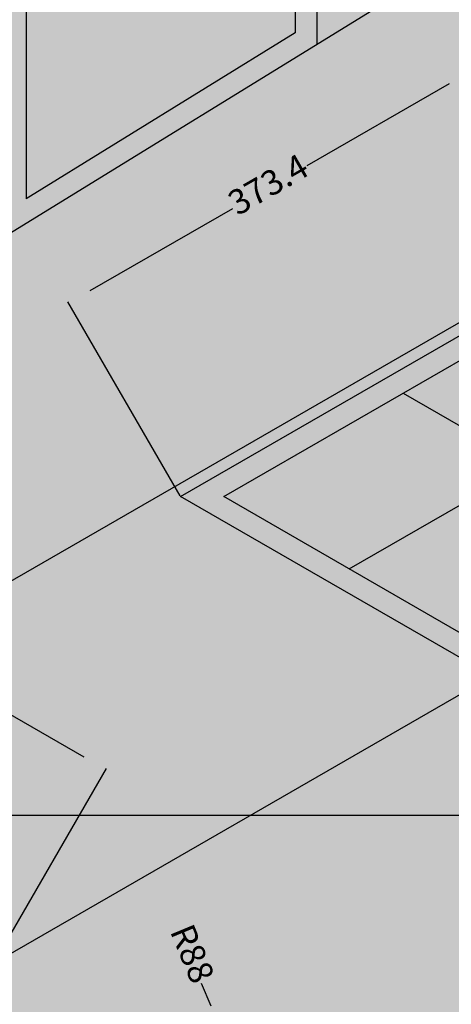
# Model space of a CAD drawing. Units: millimetres. Extents: x 78378 to 86415, y 148682 to 152721.
# Tile 3 of 18: x 78851 to 79199, y 149702 to 150495. Entities that reach past the tile are written whole.
import ezdxf

# ---------------------------------------------------------------- set-up
doc = ezdxf.new("R2010")
doc.units = ezdxf.units.MM
for name, color, linetype, lineweight in [('A-ANNO-DIMS', 2, 'Continuous', 18), ('A-FURN', 4, 'Continuous', 25), ('A-FURN-PATT', 32, 'Continuous', 13)]:
    doc.layers.add(name, color=color, linetype=linetype, lineweight=lineweight)
doc.styles.get("Standard").update_dxf_attribs({"font": 'arial.ttf'})
doc.dimstyles.new('ISO-25', dxfattribs={"dimtxt": 20, "dimasz": 20, "dimexe": 1.25, "dimexo": 0.625, "dimtad": 0, "dimdec": 1, "dimtxsty": 'Standard', "dimcen": 2.5, "dimadec": 0, "dimazin": 0, "dimtfac": 1, "dimtdec": 1, "dimtmove": 0, "dimatfit": 3, "dimfxl": 1, "dimarcsym": 0})

# ---------------------------------------------------------------- blocks, each defined once
blk = doc.blocks.new('*D19')
at = {"layer": 'A-ANNO-DIMS', "color": 0, "lineweight": -2, "transparency": 16777216}
for p, q in [((78571.17, 149885.55), (78661.48, 150041.97)), ((78678.18, 150030.89), (78771.12, 149977.23)), ((78903.35, 149900.89), (78810.4, 149954.55)), ((78830.98, 149735.55), (78921.29, 149891.97))]:
    blk.add_line(p, q, dxfattribs=at)
at = {"layer": 'A-ANNO-DIMS', "color": 0, "transparency": 16777216}
for points in [[(78679.85, 150033.78), (78676.51, 150028.01), (78660.86, 150040.89)], [(78905.01, 149903.78), (78901.68, 149898.01), (78920.67, 149890.89)]]:
    blk.add_solid(points, dxfattribs=at)
at = {"layer": 'Defpoints', "color": 0, "transparency": 16777216}
for p in [(78920.67, 149890.89), (78570.86, 149885.01), (78830.67, 149735.01)]:
    blk.add_point(p, dxfattribs=at)
at = {"layer": 'A-ANNO-DIMS', "color": 0, "transparency": 16777216, "insert": (78790.76, 149965.89), "char_height": 20, "attachment_point": 5, "rotation": 330}
blk.add_mtext('300', dxfattribs=at)
blk = doc.blocks.new('*D23')
at = {"layer": 'A-ANNO-DIMS', "color": 0, "lineweight": -2, "transparency": 16777216}
for p, q in [((79304.01, 150298.13), (79213.69, 150454.55)), ((79197, 150443.47), (79082.34, 150377.27)), ((78908.24, 150276.76), (79022.89, 150342.95)), ((78980.6, 150111.41), (78890.29, 150267.84))]:
    blk.add_line(p, q, dxfattribs=at)
at = {"layer": 'A-ANNO-DIMS', "color": 0, "transparency": 16777216}
for points in [[(79195.33, 150446.36), (79198.67, 150440.59), (79214.32, 150453.47)], [(78906.57, 150279.64), (78909.9, 150273.87), (78890.92, 150266.76)]]:
    blk.add_solid(points, dxfattribs=at)
at = {"layer": 'Defpoints', "color": 0, "transparency": 16777216}
for p in [(79214.32, 150453.47), (79304.32, 150297.59), (78980.92, 150110.87)]:
    blk.add_point(p, dxfattribs=at)
at = {"layer": 'A-ANNO-DIMS', "color": 0, "transparency": 16777216, "insert": (79052.62, 150360.11), "char_height": 20, "attachment_point": 5, "rotation": 30}
blk.add_mtext('373.4', dxfattribs=at)
blk = doc.blocks.new('*D25')
at = {"layer": 'A-ANNO-DIMS', "color": 0, "lineweight": -2, "transparency": 16777216}
for p, q in [((79360.48, 149854.03), (78389.61, 149854.03)), ((78390.86, 149834.03), (78390.86, 149656.62)), ((78390.86, 149409.86), (78390.86, 149587.28)), ((79360.48, 149389.86), (78389.61, 149389.86))]:
    blk.add_line(p, q, dxfattribs=at)
at = {"layer": 'A-ANNO-DIMS', "color": 0, "transparency": 16777216}
for points in [[(78387.53, 149834.03), (78394.19, 149834.03), (78390.86, 149854.03)], [(78387.53, 149409.86), (78394.19, 149409.86), (78390.86, 149389.86)]]:
    blk.add_solid(points, dxfattribs=at)
at = {"layer": 'Defpoints', "color": 0, "transparency": 16777216}
for p in [(78390.86, 149854.03), (79361.1, 149854.03), (79361.1, 149389.86)]:
    blk.add_point(p, dxfattribs=at)
at = {"layer": 'A-ANNO-DIMS', "color": 0, "transparency": 16777216, "insert": (78390.86, 149621.95), "char_height": 20, "attachment_point": 5, "rotation": 90}
blk.add_mtext('464.2', dxfattribs=at)
blk = doc.blocks.new('*D61')
at = {"layer": 'A-ANNO-DIMS', "color": 0, "lineweight": -2, "transparency": 16777216}
for p, q in [((79224.25, 149639.59), (79209.69, 149625.87)), ((79095.12, 149517.87), (79195.14, 149612.15))]:
    blk.add_line(p, q, dxfattribs=at)
at = {"layer": 'A-ANNO-DIMS', "color": 0, "transparency": 16777216}
blk.add_solid([(79207.41, 149628.29), (79211.98, 149623.44), (79195.14, 149612.15)], dxfattribs=at)
at = {"layer": 'Defpoints', "color": 0, "transparency": 16777216}
for p in [(79195.14, 149612.15), (79095.12, 149517.87)]:
    blk.add_point(p, dxfattribs=at)
at = {"layer": 'A-ANNO-DIMS', "color": 0, "transparency": 16777216, "insert": (79261.93, 149675.1), "char_height": 20, "attachment_point": 5, "rotation": 43.30618}
blk.add_mtext('R137.45', dxfattribs=at)
blk = doc.blocks.new('*D62')
at = {"layer": 'A-ANNO-DIMS', "color": 0, "lineweight": -2, "transparency": 16777216}
for p, q in [((78997.43, 149719.03), (79005.1, 149700.56)), ((79046.52, 149600.81), (79012.77, 149682.09))]:
    blk.add_line(p, q, dxfattribs=at)
at = {"layer": 'A-ANNO-DIMS', "color": 0, "transparency": 16777216}
blk.add_solid([(79008.18, 149701.84), (79002.02, 149699.28), (79012.77, 149682.09)], dxfattribs=at)
at = {"layer": 'Defpoints', "color": 0, "transparency": 16777216}
for p in [(79012.77, 149682.09), (79046.52, 149600.81)]:
    blk.add_point(p, dxfattribs=at)
at = {"layer": 'A-ANNO-DIMS', "color": 0, "transparency": 16777216, "insert": (78988.02, 149741.69), "char_height": 20, "attachment_point": 5, "rotation": 292.54744}
blk.add_mtext('R88', dxfattribs=at)

msp = doc.modelspace()

# ---------------------------------------------------------------- hatches: boundary and pattern name
at = {"layer": 'A-FURN-PATT'}
h = msp.add_hatch(color=256, dxfattribs=at)
h.dxf.hatch_style = 1
h.paths.add_polyline_path([(78839.3276, 151040.0076), (78579.52, 151190.0076), (78579.52, 150470.0076), (78839.3276, 150320.0076)])
h.paths.add_polyline_path([(79073.1545, 150899.6469, 0.27777969), (79002.2645, 150996.3205, 0.79108393), (78917.9567, 150978.8719, 0.18044832), (78856.6481, 150853.0138), (78856.6481, 150350.6973), (79073.1545, 150484.318)])
h.paths.add_polyline_path([(79073.1545, 151175.0076), (78856.6481, 151050.0076), (78856.6481, 150853.0138, -0.18044832), (78917.9567, 150978.8719, -0.79108393), (79002.2645, 150996.3205, -0.27777969), (79073.1545, 150899.6469)])
h.paths.add_polyline_path([(79341.6224, 151350.0076), (79099.1352, 151490.0076), (78596.8405, 151200.0076), (78839.3276, 151060.0076)])
h.paths.add_polyline_path([(79904.5389, 151675.0076), (79662.0518, 151815.0076), (79099.1352, 151490.0076), (79341.6224, 151350.0076)])
h.paths.add_polyline_path([(80389.5131, 151955.0076), (80389.5131, 152235.0076), (79662.0518, 151815.0076), (79904.5389, 151675.0076)])
h.paths.add_polyline_path([(80389.5131, 151955.0076), (80164.3465, 151825.0076), (80164.3465, 151105.0076), (80614.6797, 151105.0076), (80614.6797, 151825.0076)])
edge = h.paths.add_edge_path(flags=16)
edge.add_spline(control_points=[(80216.308, 151728.251), (80227.1854, 151732.981), (80256.3301, 151745.6544), (80298.41, 151761.9595), (80340.2597, 151805.855), (80391.0771, 151782.0404), (80454.0396, 151805.7581), (80496.5007, 151742.4095), (80543.8218, 151733.4043), (80562.7182, 151729.8083)], knot_values=[0, 0, 0, 0, 35.54374676, 95.23575347, 136.36767513, 200.93298197, 236.72641081, 322.88993498, 380.17027367, 380.17027367, 380.17027367, 380.17027367], degree=3, periodic=0)
edge.add_line((80562.7182, 151729.8083), (80562.7182, 151165.0076))
edge.add_line((80562.7182, 151165.0076), (80216.308, 151165.0076))
edge.add_line((80216.308, 151165.0076), (80216.308, 151728.251))
h.paths.add_polyline_path([(80632.0002, 152095.0076), (80389.5131, 152235.0076), (80389.5131, 151955.0076), (80614.6797, 151825.0076), (80632.0002, 151815.0076)])
h.paths.add_polyline_path([(80867.7794, 151958.8805), (80632.0002, 152095.0076), (80632.0002, 151815.0076), (80632.0002, 151510.0076), (80867.7794, 151373.8805)])
h.paths.add_polyline_path([(80147.026, 151495.8203, 0.18918979), (80063.5671, 151597.7244, 0.78826136), (79979.2691, 151580.5832, 0.16072613), (79904.5389, 151413.5769), (79904.5389, 150955.0076), (80147.026, 151095.0076)])
h.paths.add_polyline_path([(80147.026, 151815.0076), (79904.5389, 151675.0076), (79904.5389, 151413.5769, -0.16072613), (79979.2691, 151580.5832, -0.78826136), (80063.5671, 151597.7244, -0.18918979), (80147.026, 151495.8203)])
h.paths.add_polyline_path([(79887.2184, 151645.0076), (79640.4011, 151502.5076), (79640.4011, 151262.3325, -0.16072613), (79715.1313, 151429.3387, -0.78826136), (79799.4294, 151446.48, -0.21290578), (79887.2184, 151328.7247)])
h.paths.add_polyline_path([(79799.4294, 151446.48, 0.78826136), (79715.1313, 151429.3387, 0.16072613), (79640.4011, 151262.3325), (79640.4011, 150822.5076), (79887.2184, 150965.0076), (79887.2184, 151328.7247, 0.21290578)])
h.paths.add_polyline_path([(79605.7601, 151482.5076), (79358.9429, 151340.0076), (79358.9429, 151100.0701, -0.16072613), (79433.6731, 151267.0764, -0.78826136), (79517.9711, 151284.2176, -0.21290578), (79605.7601, 151166.4623)])
h.paths.add_polyline_path([(79605.7601, 151166.4623, 0.21290578), (79517.9711, 151284.2176, 0.78826136), (79433.6731, 151267.0764, 0.16072613), (79358.9429, 151100.0701), (79358.9429, 150742.9831), (79419.0877, 150694.7323), (79605.7601, 150802.5076)])
edge = h.paths.add_edge_path(flags=0)
edge.add_spline(control_points=[(81152.4356, 151098.7676), (81105.7208, 151145.9466), (81038.6136, 151213.7208), (80882.3866, 151214.1938), (80797.4434, 151311.2997), (80711.8686, 151340.3754), (80681.7691, 151350.6023)], knot_values=[0, 0, 0, 0, 188.233441, 270.4032752, 445.45179201, 540.42858829, 540.42858829, 540.42858829, 540.42858829], degree=3, periodic=0)
edge.add_line((80683.4538, 151350.0269), (80683.4538, 151104.8792))
edge.add_line((80683.4538, 151104.8792), (81152.4356, 150851.399))
edge.add_line((81152.4356, 150851.399), (81152.4356, 151098.7676))
edge = h.paths.add_edge_path(flags=0)
edge.add_spline(control_points=[(80912.9018, 151027.1103), (80892.3742, 151034.1027), (80860.1663, 151045.0739), (80835.5097, 151068.1214), (80826.5679, 151076.4797)], knot_values=[0, 0, 0, 0, 63.98405104, 100.39142428, 100.39142428, 100.39142428, 100.39142428], degree=3, periodic=0)
edge.add_arc((80830.0414, 151081.2992), 5.9407, 100.9277276, 234.2187381, ccw=False)
edge.add_spline(control_points=[(80828.9152, 151087.1322), (80837.857, 151078.7739), (80862.5136, 151055.7263), (80894.7215, 151044.7552), (80915.2491, 151037.7628)], knot_values=[0, 0, 0, 0, 36.40737324, 100.39142428, 100.39142428, 100.39142428, 100.39142428], degree=3, periodic=0)
edge.add_arc((80914.7882, 151032.2795), 5.5026, -107.9540399, 85.195579, ccw=False)
h.paths.add_polyline_path([(81238.218, 151110.0076), (80632.0002, 151460.0076), (80632.0002, 151105.0076), (81238.218, 150755.0076)])
edge = h.paths.add_edge_path(flags=16)
edge.add_line((81152.4356, 150851.399), (80683.4538, 151104.8792))
edge.add_line((80683.4538, 151104.8792), (80683.4538, 151350.0279))
edge.add_spline(control_points=[(80681.7691, 151350.6023), (80711.8686, 151340.3754), (80797.4434, 151311.2997), (80882.3866, 151214.1938), (81038.6136, 151213.7208), (81105.7208, 151145.9466), (81152.4356, 151098.7676)], knot_values=[0, 0, 0, 0, 94.97679628, 270.02531309, 352.19514729, 540.42858829, 540.42858829, 540.42858829, 540.42858829], degree=3, periodic=0)
edge.add_line((81152.4356, 151098.7676), (81152.4356, 150851.399))
edge = h.paths.add_edge_path(flags=0)
edge.add_spline(control_points=[(80912.9018, 151027.1103), (80892.3742, 151034.1027), (80860.1663, 151045.0739), (80835.5097, 151068.1214), (80826.5679, 151076.4797)], knot_values=[0, 0, 0, 0, 63.98405104, 100.39142428, 100.39142428, 100.39142428, 100.39142428], degree=3, periodic=0)
edge.add_arc((80830.0414, 151081.2992), 5.9407, 100.9277276, 234.2187381, ccw=False)
edge.add_spline(control_points=[(80828.9152, 151087.1322), (80837.857, 151078.7739), (80862.5136, 151055.7263), (80894.7215, 151044.7552), (80915.2491, 151037.7628)], knot_values=[0, 0, 0, 0, 36.40737324, 100.39142428, 100.39142428, 100.39142428, 100.39142428], degree=3, periodic=0)
edge.add_arc((80914.7882, 151032.2795), 5.5026, -107.7417882, 85.195579, ccw=False)
h.paths.add_polyline_path([(81498.0256, 151255.0076), (81238.218, 151110.0076), (81238.218, 150755.0076), (81498.0256, 150905.0076)])
edge = h.paths.add_edge_path(flags=16)
edge.add_spline(control_points=[(81152.4356, 151098.7676), (81105.7208, 151145.9466), (81038.6136, 151213.7208), (80882.3866, 151214.1938), (80797.4434, 151311.2997), (80711.8686, 151340.3754), (80681.7691, 151350.6023)], knot_values=[0, 0, 0, 0, 188.233441, 270.4032752, 445.45179201, 540.42858829, 540.42858829, 540.42858829, 540.42858829], degree=3, periodic=0)
edge.add_line((80683.4538, 151350.0279), (80683.4538, 151104.8792))
edge.add_line((80683.4538, 151104.8792), (81152.4356, 150851.399))
edge.add_line((81152.4356, 150851.399), (81152.4356, 151098.7676))
h.paths.add_polyline_path([(81453.9904, 151280.4314), (80867.7794, 151618.8805), (80867.7794, 151373.8805), (81238.218, 151160.0076)])
edge = h.paths.add_edge_path(flags=16)
edge.add_line((81189.2304, 151297.6373), (81114.4166, 151300.2154))
edge.add_arc((81412.0967, 151394.0167), 312.1092, 179.7569303, 197.4900342, ccw=False)
edge.add_ellipse((81154.0183, 151392.0436), major_axis=(-54.0264, 3.6301), ratio=0.22179693, start_angle=0, end_angle=0.3517985, ccw=False)
edge.add_ellipse((81154.0183, 151392.0436), major_axis=(-54.0264, 3.6301), ratio=0.22179693, start_angle=180, end_angle=360, ccw=False)
edge.add_spline(control_points=[(81196.1844, 151321.9476), (81224.9802, 151347.1455), (81266.8846, 151383.8144), (81222.0354, 151387.0304), (81208.0056, 151388.0364)], knot_values=[0, 0, 0, 0, 75.09175173, 109.27580439, 109.27580439, 109.27580439, 109.27580439], degree=3, periodic=0)
edge.add_arc((80751.9112, 151435.6145), 458.5693, 342.4891602, 345.646172, ccw=False)
edge = h.paths.add_edge_path(flags=0)
edge.add_spline(control_points=[(81196.6193, 151323.657), (81197.893, 151324.7717), (81199.1654, 151325.8858), (81209.0233, 151334.5343), (81217.3959, 151341.9835), (81228.0928, 151352.5012), (81231.3883, 151355.9524), (81236.9493, 151362.4395), (81239.214, 151365.4773), (81241.4987, 151369.416), (81242.064, 151370.5542), (81242.9187, 151372.6971), (81243.2076, 151373.7015), (81243.5012, 151375.5539), (81243.5065, 151376.4), (81243.2432, 151377.9407), (81242.9775, 151378.6373), (81242.1402, 151379.937), (81241.5659, 151380.5416), (81240.2039, 151381.533), (81239.4963, 151381.9384), (81237.0619, 151383.0663), (81235.0242, 151383.6999), (81230.352, 151384.7569), (81227.7173, 151385.1826), (81221.9118, 151385.9145), (81218.7193, 151386.2133), (81213.7912, 151386.6115), (81212.1252, 151386.7359), (81209.6196, 151386.9181), (81208.7865, 151386.9779), (81207.9009, 151387.0432)], knot_values=[0.01548744, 0.01548744, 0.01548744, 0.01548744, 3.33787957, 3.33787957, 25.85130624, 25.85130624, 37.52811308, 37.52811308, 49.20491992, 49.20491992, 54.2850938, 54.2850938, 59.36526768, 59.36526768, 64.44544157, 64.44544157, 69.52561545, 69.52561545, 74.60578933, 74.60578933, 78.49366785, 78.49366785, 86.25567095, 86.25567095, 94.01767406, 94.01767406, 102.20226556, 102.20226556, 106.29456131, 106.29456131, 108.32522175, 108.32522175, 108.32522175, 108.32522175], degree=3, periodic=0)
edge = h.paths.add_edge_path(flags=16)
edge.add_arc((81034.1732, 151350.4693), 42.5822, 231.2679035, 306.151846, ccw=False)
edge.add_line((81007.5303, 151317.2517), (81007.5303, 151395.181))
edge.add_ellipse((81033.412, 151394.7791), major_axis=(-25.8816, 0.4538), ratio=0.23894509, start_angle=0, end_angle=0.1147075, ccw=False)
edge.add_ellipse((81033.412, 151394.7791), major_axis=(-25.8816, 0.4538), ratio=0.23894509, start_angle=181.1677709, end_angle=358.9476457, ccw=False)
edge.add_ellipse((81033.412, 151395.7791), major_axis=(-25.8816, 0.4538), ratio=0.23894509, start_angle=180, end_angle=360.1147075, ccw=False)
edge.add_ellipse((81033.412, 151395.7791), major_axis=(-25.8816, 0.4538), ratio=0.23894509, start_angle=178.9476457, end_angle=180, ccw=False)
edge.add_line((81059.2936, 151395.1778), (81059.2936, 151394.3772))
edge.add_ellipse((81033.412, 151394.7791), major_axis=(-25.8816, 0.4538), ratio=0.23894509, start_angle=180, end_angle=180.1147075, ccw=False)
edge.add_ellipse((81033.412, 151394.7791), major_axis=(-25.8816, 0.4538), ratio=0.23894509, start_angle=3.6903098, end_angle=176.4406503, ccw=False)
edge.add_line((81059.2936, 151393.3388), (81059.2936, 151316.086))
h.paths.add_polyline_path([(80951.9355, 151343.9568), (80909.6838, 151362.4635), (80904.0219, 151443.9615, -0.38133308), (80987.2169, 151411.3717)], flags=16)
h = msp.add_hatch(color=256, dxfattribs=at)
h.dxf.hatch_style = 1
h.paths.add_polyline_path([(80389.8136, 150935.1811), (80389.5131, 151105.0076), (80164.3465, 151105.0076), (79904.5389, 150955.0076), (79433.5848, 150683.1022), (79459.4128, 150662.3818), (79243.9048, 150537.9582), (79160.4069, 150518.1674), (78839.3276, 150320.0076), (78579.52, 150470.0076), (78570.8597, 150475.0076), (78570.8597, 150465.0076), (78570.8597, 149885.0076)])
h.paths.add_polyline_path([(80086.4042, 150460.0076), (79826.5966, 150610.0076), (78570.8597, 149885.0076), (78830.6674, 149735.0076)])
h.paths.add_polyline_path([(79540.8001, 150161.0557), (79217.3967, 149974.3386), (78980.9166, 150110.8705), (79304.32, 150297.5875)], flags=16)
h.paths.add_polyline_path([(79506.159, 150161.0557), (79217.3967, 149994.3386), (79015.5576, 150110.8705), (79304.32, 150277.5875)], flags=0)
edge = h.paths.add_edge_path(flags=0)
edge.add_arc((79247.8636, 150177.1541), 137.9799, 256.0025928, 293.5594109)
edge.add_arc((79240.7671, 150078.2605), 68.0855, 336.099104, 387.3696877)
edge.add_ellipse((79258.3074, 150109.4852), major_axis=(-42.6234, -1.6591), ratio=0.16042843, start_angle=0, end_angle=179.0977279, ccw=False)
edge.add_arc((79285.2112, 150074.2509), 77.2096, 155.1233104, 203.6557939)
edge = h.paths.add_edge_path(flags=0)
edge.add_ellipse((79258.6958, 150110.8297), major_axis=(-42.6234, -1.6591), ratio=0.16042843, start_angle=350.6039412, end_angle=356.2289762)
edge.add_line((79219.169, 150111.8937), (79218.3268, 150109.4141))
edge.add_arc((79262.4675, 150032.9602), 88.2813, 112.3931229, 120, ccw=False)
h.paths.add_polyline_path([(79287.0625, 150086.9703, -0.24770206), (79288.1967, 150077.2955, -0.39047651), (79265.4731, 150072.5438, -0.48726153), (79264.079, 150082.3769, 0.39560433)], flags=0)
h.paths.add_polyline_path([(80389.5131, 150935.0076), (79826.5966, 150610.0076), (80086.4042, 150460.0076), (80692.622, 150460.0076), (80952.4296, 150610.0076)])
edge = h.paths.add_edge_path(flags=16)
edge.add_ellipse((80392.4466, 150825.601), major_axis=(-133.0757, 7.722), ratio=0.42449957, start_angle=0, end_angle=360)
edge = h.paths.add_edge_path(flags=0)
edge.add_spline(control_points=[(80269.3541, 150832.7436), (80269.2919, 150831.672), (80269.3503, 150830.5922), (80269.7341, 150828.3361), (80270.0612, 150827.1587), (80271.0461, 150824.6748), (80271.7052, 150823.3692), (80273.4061, 150820.6503), (80274.4481, 150819.2381), (80276.9366, 150816.3509), (80278.3828, 150814.8762), (80282.5858, 150811.0913), (80285.6261, 150808.7701), (80292.6031, 150804.2267), (80296.5388, 150802.0041), (80305.195, 150797.7581), (80309.9151, 150795.7344), (80320.0112, 150791.96), (80325.387, 150790.2092), (80339.2162, 150786.315), (80347.9578, 150784.3563), (80366.0679, 150781.2568), (80375.4359, 150780.1158), (80394.3093, 150778.7158), (80403.8142, 150778.4568), (80422.4656, 150778.8319), (80431.6115, 150779.4662), (80449.0608, 150781.5838), (80457.3636, 150783.0675), (80472.6699, 150786.7766), (80479.6726, 150789.0033), (80490.1894, 150793.2813), (80494.1268, 150795.1967), (80501.0146, 150799.1885), (80503.9632, 150801.2651), (80508.2066, 150804.9015), (80509.73, 150806.4609), (80512.1996, 150809.4942), (80513.1456, 150810.9657), (80514.4291, 150813.5431), (80514.8436, 150814.6688), (80515.3984, 150816.8625), (80515.5405, 150817.9315), (80515.5801, 150820.098), (80515.4773, 150821.1978), (80514.9905, 150823.5062), (80514.6047, 150824.7154), (80513.4854, 150827.2641), (80512.7511, 150828.6027), (80510.8872, 150831.3809), (80509.7578, 150832.8196), (80507.0873, 150835.7513), (80505.5466, 150837.2439), (80501.0624, 150841.0944), (80497.8199, 150843.4576), (80490.4174, 150848.062), (80486.2582, 150850.3037), (80477.1448, 150854.5643), (80472.1909, 150856.5835), (80461.6275, 150860.3245), (80456.0182, 150862.0465), (80441.7332, 150865.8127), (80432.7885, 150867.6675), (80414.3391, 150870.5317), (80404.8349, 150871.5411), (80385.7707, 150872.6572), (80376.2113, 150872.764), (80357.5444, 150872.0728), (80348.4375, 150871.2748), (80331.1682, 150868.83), (80323.0064, 150867.1827), (80309.472, 150863.5363), (80303.8628, 150861.6593), (80293.8018, 150857.5401), (80289.3512, 150855.2969), (80282.7757, 150851.2345), (80280.3473, 150849.4579), (80276.2606, 150845.9127), (80274.604, 150844.1458), (80272.3157, 150841.1243), (80271.5358, 150839.8454), (80270.3496, 150837.3879), (80269.9417, 150836.2101), (80269.5065, 150834.2815), (80269.3988, 150833.5143), (80269.3541, 150832.7436)], knot_values=[0, 0, 0, 0, 0.09750046, 0.09750046, 0.19500092, 0.19500092, 0.29250138, 0.29250138, 0.39000184, 0.39000184, 0.4875023, 0.4875023, 0.63880322, 0.63880322, 0.79010415, 0.79010415, 0.94140507, 0.94140507, 1.092706, 1.092706, 1.3128171, 1.3128171, 1.5329282, 1.5329282, 1.7530393, 1.7530393, 1.97315041, 1.97315041, 2.19326151, 2.19326151, 2.41337261, 2.41337261, 2.56986063, 2.56986063, 2.72634866, 2.72634866, 2.84418658, 2.84418658, 2.96202451, 2.96202451, 3.06023388, 3.06023388, 3.15844325, 3.15844325, 3.25665261, 3.25665261, 3.35486198, 3.35486198, 3.45307135, 3.45307135, 3.55128072, 3.55128072, 3.64949009, 3.64949009, 3.80392773, 3.80392773, 3.95836537, 3.95836537, 4.11280301, 4.11280301, 4.26724064, 4.26724064, 4.48920349, 4.48920349, 4.71116635, 4.71116635, 4.9331292, 4.9331292, 5.15509205, 5.15509205, 5.3770549, 5.3770549, 5.55785361, 5.55785361, 5.73865232, 5.73865232, 5.87239556, 5.87239556, 6.00613879, 6.00613879, 6.109605, 6.109605, 6.2130712, 6.2130712, 6.28318531, 6.28318531, 6.28318531, 6.28318531], degree=3, periodic=0)
edge = h.paths.add_edge_path(flags=0)
edge.add_ellipse((80392.4466, 150825.601), major_axis=(-101.8398, 3.3923), ratio=0.40349248, start_angle=0, end_angle=360)
edge = h.paths.add_edge_path(flags=0)
edge.add_ellipse((80391.1657, 150858.3746), major_axis=(9.0882, -0.6733), ratio=0.35135413, start_angle=0, end_angle=360)
h.paths.add_polyline_path([(80952.4296, 150610.0076), (80692.622, 150460.0076), (81361.2342, 150073.9842), (81649.9628, 150052.7286), (81766.4935, 150120.0076), (81766.4935, 150140.0076), (81564.9025, 150256.3963), (81564.8884, 150096.1963), (81538.9076, 150111.1963), (81538.9217, 150271.3963)])
h.paths.add_polyline_path([(81539.0357, 151571.3305), (80867.7794, 151958.8805), (80867.7794, 151618.8805), (81498.0256, 151255.0076), (81498.0256, 150905.0076), (81238.218, 150755.0076), (81538.9488, 150581.3806)])
h.paths.add_polyline_path([(81766.4935, 151440.0076), (81565.0164, 151556.3305), (81564.9296, 150566.3806), (81766.4935, 150450.0076)])
edge = h.paths.add_edge_path()
edge.add_line((81564.9296, 150566.3806), (81564.9137, 150384.6289))
edge.add_ellipse((81552.1304, 150358.5718), major_axis=(52.6272, 3.506), ratio=0.49589905, start_angle=367.5169757, end_angle=420.0564686, ccw=False)
edge.add_ellipse((81552.1304, 150358.5718), major_axis=(52.6272, 3.506), ratio=0.49589905, start_angle=351.729742, end_angle=367.5169757, ccw=False)
edge.add_ellipse((81552.1304, 150345.5016), major_axis=(52.6272, 3.506), ratio=0.49589905, start_angle=352.5116949, end_angle=366.3006092, ccw=False)
edge.add_line((81603.4463, 150342.2039), (81603.5064, 150340.4475))
edge.add_ellipse((81552.1304, 150332.128), major_axis=(52.6272, 3.506), ratio=0.49589905, start_angle=353.6729654, end_angle=365.3867997, ccw=False)
edge.add_ellipse((81552.1304, 150332.128), major_axis=(52.6272, 3.506), ratio=0.49589905, start_angle=350.9388331, end_angle=353.6729654)
edge.add_line((81603.8688, 150329.855), (81604.0442, 150324.7302))
edge.add_ellipse((81552.1304, 150317.7418), major_axis=(52.6272, 3.506), ratio=0.49589905, start_angle=355.2176746, end_angle=363.8553364, ccw=False)
edge.add_ellipse((81552.1304, 150317.7418), major_axis=(52.6272, 3.506), ratio=0.49589905, start_angle=341.3250873, end_angle=355.2176746, ccw=False)
edge.add_ellipse((81552.1304, 150317.7418), major_axis=(52.6272, 3.506), ratio=0.49589905, start_angle=293.4661701, end_angle=341.3250873, ccw=False)
edge.add_line((81564.9057, 150292.9664), (81564.9025, 150256.3963))
edge.add_line((81564.9025, 150256.3963), (81766.4935, 150140.0076))
edge.add_line((81766.4935, 150140.0076), (81766.4935, 150450.0076))
edge.add_line((81766.4935, 150450.0076), (81564.9296, 150566.3806))
h.paths.add_polyline_path([(81525.5713, 150321.598), (81526.5985, 150321.3069), (81528.6771, 150320.947)])
h.paths.add_polyline_path([(81512.7903, 150326.1129), (81514.5058, 150325.3887), (81512.538, 150326.2678)])
h.paths.add_polyline_path([(81533.2148, 150320.1615), (81534.6952, 150319.9052), (81536.5995, 150319.7557)])
h.paths.add_polyline_path([(81518.622, 150323.6513), (81519.227, 150323.3959), (81521.289, 150322.8116)])
h.paths.add_polyline_path([(81501.2183, 150336.2599), (81500.3543, 150338.1339), (81499.7815, 150340.0494), (81499.5032, 150341.9955), (81499.5032, 150343.7257), (81499.7584, 150345.5905), (81500.2766, 150347.4549), (81501.0551, 150349.3095), (81501.0967, 150349.3937), (81501.1389, 150349.4778), (81500.9978, 150349.7496), (81500.8628, 150350.0225), (81499.5032, 150355.0658), (81499.9591, 150359.5002), (81501.8982, 150363.9083), (81505.2653, 150368.1646), (81509.9647, 150372.1482), (81515.8627, 150375.7459), (81522.7918, 150378.8553), (81530.555, 150381.3882), (81538.9315, 150383.2724), (81538.9488, 150581.3806), (80632.0002, 151105.0076), (80389.5131, 151105.0076), (80389.8142, 150934.8338), (80952.4296, 150610.0076), (81538.9217, 150271.3963), (81538.9234, 150291.7194), (81538.8752, 150291.721), (81530.1915, 150292.8239), (81522.1802, 150294.6904), (81515.0866, 150297.2633), (81509.8635, 150299.9959), (81505.6084, 150303.1351), (81502.419, 150306.6088), (81500.3683, 150310.3375), (81499.5032, 150314.2358), (81499.5032, 150315.9659), (81499.8206, 150318.1159), (81500.487, 150320.2634), (81501.4979, 150322.3941), (81500.487, 150324.4233), (81499.8206, 150326.5039), (81499.5032, 150328.622), (81499.5032, 150330.3521), (81499.7815, 150332.3262), (81500.3543, 150334.2992)])
h = msp.add_hatch(color=256, dxfattribs=at)
h.dxf.hatch_style = 1
h.paths.add_polyline_path([(79090.475, 151205.0076), (78839.3276, 151060.0076), (78839.3276, 150320.0076), (79090.475, 150475.0076)])
h.paths.add_polyline_path([(79073.1545, 151175.0076), (79073.1545, 150899.6469, -0.04544363), (79073.1545, 150878.5653), (79073.1545, 150484.318), (78856.6481, 150350.6973), (78856.6481, 150814.5249, -0.04815716), (78856.6481, 150853.0138), (78856.6481, 151050.0076)], flags=16)
h.paths.add_polyline_path([(79358.9429, 151340.0076), (79605.7601, 151482.5076), (79605.7601, 150802.5076), (79419.0877, 150694.7323), (79433.5848, 150683.1022), (79623.0806, 150792.5076), (79623.0806, 151512.5076), (79341.6224, 151350.0076), (79341.6224, 150756.8784), (79358.9429, 150742.9831)])
h.paths.add_polyline_path([(79341.6224, 151350.0076), (79090.475, 151205.0076), (79090.475, 150475.0076), (79160.4069, 150518.1674), (79107.7955, 150505.6973), (79107.7955, 151195.0076), (79109.5275, 151196.0076), (79324.3018, 151320.0076), (79324.3018, 150770.7736), (79341.6224, 150756.8784)])
h.paths.add_polyline_path([(79887.2184, 151645.0076), (79887.2184, 151665.0076), (79623.0806, 151512.5076), (79623.0806, 150792.5076), (79887.2184, 150945.0076), (79887.2184, 150965.0076), (79640.4011, 150822.5076), (79640.4011, 151502.5076)])
h.paths.add_polyline_path([(79904.5389, 151655.0076), (79887.2184, 151645.0076), (79887.2184, 150965.0076), (79904.5389, 150975.0076)])
h.paths.add_polyline_path([(80164.3465, 151825.0076), (80147.026, 151815.0076), (80147.026, 151095.0076), (80164.3465, 151105.0076)])
h.paths.add_polyline_path([(80632.0002, 151510.0076), (80632.0002, 151490.0076), (81238.218, 151140.0076), (81471.6045, 151270.2619), (81453.9904, 151280.4314), (81238.218, 151160.0076)])
h.paths.add_polyline_path([(80632.0002, 151490.0076), (80632.0002, 151470.0076), (81238.218, 151120.0076), (81489.2186, 151260.0924), (81471.6045, 151270.2619), (81238.218, 151140.0076)])
h.paths.add_polyline_path([(80632.0002, 151460.0076), (80632.0002, 151105.0076), (81238.218, 150755.0076), (81238.218, 151110.0076)])
edge = h.paths.add_edge_path(flags=16)
edge.add_spline(control_points=[(80681.7691, 151350.6023), (80711.8686, 151340.3754), (80797.4434, 151311.2997), (80882.3866, 151214.1938), (81038.6136, 151213.7208), (81105.7208, 151145.9466), (81152.4356, 151098.7676)], knot_values=[0, 0, 0, 0, 94.97679628, 270.02531309, 352.19514729, 540.42858829, 540.42858829, 540.42858829, 540.42858829], degree=3, periodic=0)
edge.add_line((81152.4356, 151098.7676), (81152.4356, 150851.399))
edge.add_line((81152.4356, 150851.399), (80683.4538, 151104.8792))
edge.add_line((80683.4538, 151104.8792), (80683.4538, 151350.027))
edge = h.paths.add_edge_path(flags=0)
edge.add_spline(control_points=[(80828.9152, 151087.1322), (80837.857, 151078.7739), (80862.5136, 151055.7263), (80894.7215, 151044.7552), (80915.2491, 151037.7628)], knot_values=[0, 0, 0, 0, 36.40737324, 100.39142428, 100.39142428, 100.39142428, 100.39142428], degree=3, periodic=0)
edge.add_arc((80914.7882, 151032.2795), 5.5026, -107.9540399, 85.195579, ccw=False)
edge.add_spline(control_points=[(80912.9018, 151027.1103), (80892.3742, 151034.1027), (80860.1663, 151045.0739), (80835.5097, 151068.1214), (80826.5679, 151076.4797)], knot_values=[0, 0, 0, 0, 63.98405104, 100.39142428, 100.39142428, 100.39142428, 100.39142428], degree=3, periodic=0)
edge.add_arc((80830.0414, 151081.2992), 5.9407, 100.9277276, 234.2187381, ccw=False)
h.paths.add_polyline_path([(80632.0002, 151815.0076), (80614.6797, 151825.0076), (80614.6797, 151105.0076), (80632.0002, 151105.0076)])
h.paths.add_polyline_path([(81498.0256, 151255.0076), (81489.2186, 151260.0924), (81238.218, 151120.0076), (80632.0002, 151470.0076), (80632.0002, 151460.0076), (81238.218, 151110.0076)])
h.paths.add_polyline_path([(78596.8405, 151200.0076), (78579.52, 151190.0076), (78839.3276, 151040.0076), (78839.3276, 151060.0076)])
h.paths.add_polyline_path([(78596.8405, 151200.0076), (78579.52, 151210.0076), (78579.52, 151190.0076)])
h.paths.add_polyline_path([(78579.52, 151210.0076), (78570.8597, 151205.0076), (78570.8597, 150475.0076), (78579.52, 150470.0076)])
h = msp.add_hatch(color=256, dxfattribs=at)
h.dxf.hatch_style = 1
h.paths.add_polyline_path([(79304.32, 150297.5875), (78980.9166, 150110.8705), (79217.3967, 149974.3386), (79540.8001, 150161.0557)])
h.paths.add_polyline_path([(79506.159, 150161.0557), (79217.3967, 149994.3386), (79015.5576, 150110.8705), (79304.32, 150277.5875)], flags=16)
edge = h.paths.add_edge_path(flags=0)
edge.add_line((79260.8583, 150135.9631), (79296.366, 150115.4627))
edge.add_ellipse((79258.6958, 150110.8297), major_axis=(-42.6234, -1.6591), ratio=0.16042843, start_angle=540.1624997, end_angle=544.7822411, ccw=False)
edge.add_ellipse((79258.6958, 150110.8297), major_axis=(-42.6234, -1.6591), ratio=0.16042843, start_angle=540, end_angle=540.1624997, ccw=False)
edge.add_line((79301.3113, 150112.6075), (79301.4117, 150112.5496))
edge.add_ellipse((79258.6958, 150110.8297), major_axis=(-42.6234, -1.6591), ratio=0.16042843, start_angle=538.60644, end_angle=539.6688473, ccw=False)
edge.add_arc((79299.1378, 150112.0107), 2.2333, -43.6788662, 8.9937503, ccw=False)
edge.add_arc((79240.7671, 150078.2605), 68.0855, -23.900896, 28.2323958, ccw=False)
edge.add_arc((79247.8636, 150177.1541), 137.9799, 256.0025928, 293.5594109, ccw=False)
edge.add_arc((79285.2112, 150074.2509), 77.2096, 154.2238314, 203.6557939, ccw=False)
edge.add_ellipse((79258.3074, 150109.4852), major_axis=(-42.6234, -1.6591), ratio=0.16042843, start_angle=359.9882645, end_angle=360, ccw=False)
edge.add_arc((79216.8461, 150108.3941), 1.2901, 125.5884183, 205.6940851, ccw=False)
edge.add_ellipse((79258.6958, 150110.8297), major_axis=(-42.6234, -1.6591), ratio=0.16042843, start_angle=358.1218837, end_angle=359.634987, ccw=False)
edge.add_line((79216.51, 150110.3586), (79216.8824, 150110.5736))
edge.add_ellipse((79258.6958, 150110.8297), major_axis=(-42.6234, -1.6591), ratio=0.16042843, start_angle=356.2289762, end_angle=358.1218837, ccw=False)
edge.add_line((79219.169, 150111.8937), (79260.8583, 150135.9631))
h.paths.add_polyline_path([(79288.1967, 150077.2955, -0.39047651), (79265.4731, 150072.5438, -0.48726153), (79264.079, 150082.3769, 0.39560433), (79287.0625, 150086.9703, -0.24770206)], flags=0)
h = msp.add_hatch(color=256, dxfattribs=at)
h.dxf.hatch_style = 1
edge = h.paths.add_edge_path()
edge.add_line((79506.159, 150161.0557), (79405.2395, 150219.3216))
edge.add_line((79405.2395, 150219.3216), (79260.8583, 150135.9631))
edge.add_line((79260.8583, 150135.9631), (79296.366, 150115.4627))
edge.add_ellipse((79258.6958, 150110.8297), major_axis=(-42.6234, -1.6591), ratio=0.16042843, start_angle=540.1624997, end_angle=544.7822411, ccw=False)
edge.add_ellipse((79258.6958, 150110.8297), major_axis=(-42.6234, -1.6591), ratio=0.16042843, start_angle=538.60644, end_angle=539.6688473, ccw=False)
edge.add_line((79301.4117, 150112.5496), (79361.7779, 150077.6971))
edge.add_line((79361.7779, 150077.6971), (79506.159, 150161.0557))
h.paths.add_polyline_path([(79405.2395, 150219.3216), (79304.32, 150277.5875), (79159.9388, 150194.229), (79260.8583, 150135.9631)])
edge = h.paths.add_edge_path()
edge.add_line((79260.8583, 150135.9631), (79159.9388, 150194.229))
edge.add_line((79159.9388, 150194.229), (79015.5576, 150110.8705))
edge.add_line((79015.5576, 150110.8705), (79116.4771, 150052.6045))
edge.add_line((79116.4771, 150052.6045), (79216.8824, 150110.5736))
edge.add_ellipse((79258.6958, 150110.8297), major_axis=(-42.6234, -1.6591), ratio=0.16042843, start_angle=356.2289762, end_angle=358.1218837, ccw=False)
edge.add_ellipse((79258.6958, 150110.8297), major_axis=(-42.6234, -1.6591), ratio=0.16042843, start_angle=350.6039412, end_angle=356.2289762)
edge.add_line((79219.169, 150111.8937), (79260.8583, 150135.9631))
h.paths.add_polyline_path([(79300.7529, 150110.4683, 0.21642229), (79301.362, 150112.2118, 0.25927743), (79215.6839, 150107.826, 0.21909574), (79214.4893, 150043.2712, 0.16535535), (79303.0141, 150050.6753, 0.23148087)], flags=16)
h.paths.add_polyline_path([(79264.079, 150082.3769, 0.39560433), (79287.0625, 150086.9703, -0.24770206), (79288.1967, 150077.2955, -0.39047651), (79265.4731, 150072.5438, -0.48726153)], flags=0)
h.paths.add_polyline_path([(79361.7779, 150077.6971), (79301.4117, 150112.5496), (79260.8583, 150135.9631), (79116.4771, 150052.6045), (79217.3967, 149994.3386)])
edge = h.paths.add_edge_path(flags=16)
edge.add_ellipse((79258.3074, 150109.4852), major_axis=(-42.6234, -1.6591), ratio=0.16042843, start_angle=180.4067093, end_angle=238.2058938, ccw=False)
edge.add_arc((79299.1378, 150112.0107), 2.2333, 335.7071144, 365.168126)
edge.add_arc((79262.4675, 150032.9602), 88.2813, 63.8595099, 90.1998686)
edge.add_arc((79256.9649, 150118.7368), 5.7667, -23.3220096, 25.7370753, ccw=False)
edge = h.paths.add_edge_path(flags=0)
edge.add_ellipse((79258.3074, 150109.4852), major_axis=(-42.6234, -1.6591), ratio=0.16042843, start_angle=0, end_angle=179.0977279, ccw=False)
edge.add_arc((79285.2112, 150074.2509), 77.2096, 154.2238314, 203.6557939)
edge.add_arc((79247.8636, 150177.1541), 137.9799, 256.0025928, 293.5594109)
edge.add_arc((79240.7671, 150078.2605), 68.0855, 336.099104, 388.2323958)
h = msp.add_hatch(color=256, dxfattribs=at)
h.dxf.hatch_style = 1
h.paths.add_polyline_path([(78830.6674, 149715.0076), (78570.8597, 149865.0076), (78570.8597, 149055.0076), (78830.6674, 148905.0076)])
h.paths.add_polyline_path([(79257.8556, 149981.6449), (78830.6674, 149735.0076), (78830.6674, 148905.0076), (79257.8556, 149151.6449)])
h.paths.add_polyline_path([(79116.9453, 149653.5787, -0.33999439), (79231.8748, 149531.6449), (79231.8748, 149166.6449), (78856.6481, 148950.0076), (78856.6481, 149398.1143, -0.25342364), (78959.4208, 149588.1766, -0.77714453)], flags=16)
h.paths.add_polyline_path([(79231.8748, 149531.6449, 0.33999439), (79116.9453, 149653.5787, 0.77714453), (78959.4208, 149588.1766, 0.25342364), (78856.6481, 149398.1143), (78856.6481, 148950.0076), (79231.8748, 149166.6449)], flags=0)

# ---------------------------------------------------------------- linework, layer by layer
at = {"layer": 'A-FURN'}
for p, q in [((79090.475, 151205.0076), (79090.475, 150475.0076)), ((79073.1545, 151175.0076), (79073.1545, 150484.318)), ((78856.6481, 151050.0076), (78856.6481, 150350.6973)), ((78570.8597, 149885.0076), (80389.5131, 150935.0076)), ((79160.4069, 150518.1674), (78839.3276, 150320.0076)), ((79073.1545, 150484.318), (78856.6481, 150350.6973)), ((78830.6674, 149735.0076), (80086.4042, 150460.0076)), ((78980.9166, 150110.8705), (79304.32, 150297.5875)), ((79015.5576, 150110.8705), (79304.32, 150277.5875)), ((79116.4771, 150052.6045), (79405.2395, 150219.3216)), ((79159.9388, 150194.229), (79361.7779, 150077.6971)), ((79217.4042, 149974.3343), (78980.9166, 150110.8705)), ((79217.3967, 149994.3386), (79015.5576, 150110.8705))]:
    msp.add_line(p, q, dxfattribs=at)

# ---------------------------------------------------------------- dimensions: what is measured, and where the dimension line sits
at = {"layer": 'A-ANNO-DIMS'}
for base, p1, p2, angle, override, picture, middle in [((79214.32, 150453.4721), (78980.9166, 150110.8705), (79304.32, 150297.5875), 30, {"dimdec": 1, "dimlfac": 1, "dimrnd": 0, "dimzin": 0, "dimdsep": 46, "dimlunit": 2}, '*D23', (79052.6183, 150360.1136)), ((78920.6674, 149890.8922), (78570.8597, 149885.0076), (78830.6674, 149735.0076), 330, {"dimdec": 0, "dimlfac": 1, "dimrnd": 0, "dimzin": 0, "dimdsep": 46, "dimlunit": 2}, '*D19', (78790.7636, 149965.8922)), ((78390.8597, 149854.0252), (79361.1019, 149389.8649), (79361.1019, 149854.0252), 90, {"dimdec": 1, "dimlfac": 1, "dimrnd": 0, "dimzin": 0, "dimdsep": 46, "dimlunit": 2}, '*D25', (78390.8597, 149621.945))]:
    dim = msp.add_linear_dim(base=base, p1=p1, p2=p2, angle=angle, dimstyle='ISO-25', override=override, dxfattribs=at)
    dim.commit()
    dim.dimension.update_dxf_attribs({"geometry": picture, "text_midpoint": middle})
for center, mpoint, override, picture, middle in [((79046.5156, 149600.8083), (79012.7698, 149682.0874), {"dimdec": 0, "dimlfac": 1, "dimrnd": 0, "dimzin": 0, "dimdsep": 46, "dimlunit": 2}, '*D62', (78988.0219, 149741.6945)), ((79095.1156, 149517.8722), (79195.1385, 149612.1495), {"dimdec": 2, "dimlfac": 1, "dimrnd": 0, "dimzin": 0, "dimdsep": 46, "dimlunit": 2}, '*D61', (79261.9301, 149675.1043))]:
    dim = msp.add_radius_dim(center=center, mpoint=mpoint, dimstyle='ISO-25', override=override, dxfattribs=at)
    dim.commit()
    dim.dimension.update_dxf_attribs({"geometry": picture, "text_midpoint": middle})

doc.saveas('drawing.dxf')
